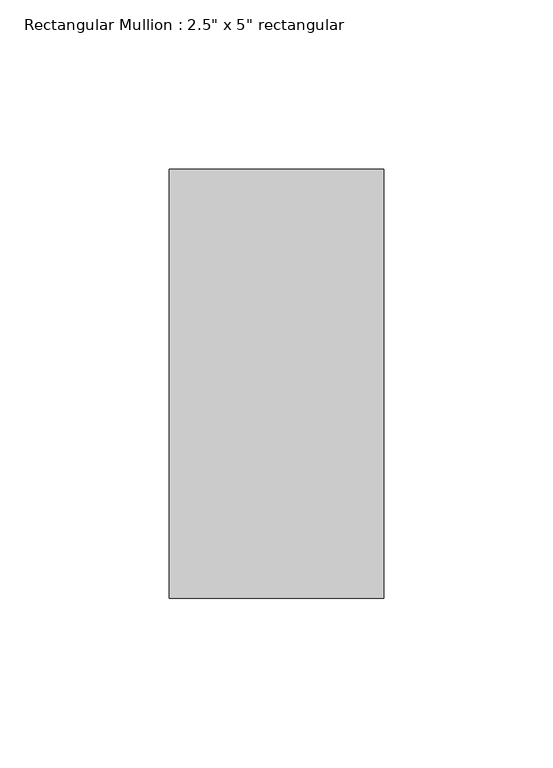
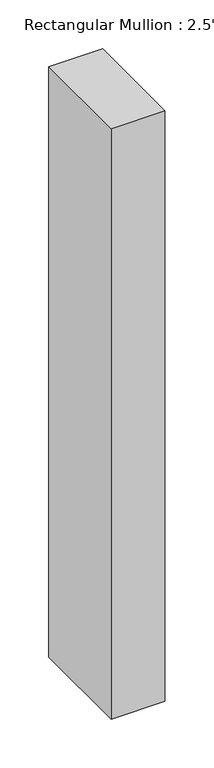
"""IFC4 building model written with IfcOpenShell, lengths in millimetres: member geometry."""

from ifc_helpers import new_model, si_unit, frame, origin, place, context, project, spatial, polyline, outline, extrude, source, transform, mapped, element, save


def member_8ca7f02a(model_context):
    return source(origin(), model_context, "Body", "SweptSolid", [
        extrude(outline(polyline([(31.75, 63.5), (31.75, -63.5), (-31.75, -63.5), (-31.75, 63.5), (31.75, 63.5)])), frame((0.0, 0.0, -736.6), z_axis=(0.0, 0.0, 1.0), x_axis=(1.0, 0.0, 0.0)), (0.0, 0.0, 1.0), 736.6),
    ])


if __name__ == "__main__":
    model = new_model("IFC4")
    model_context = context("Model", 3, world=origin())
    ifc_project = project(units=[si_unit("LENGTHUNIT", "METRE", prefix="MILLI")], contexts=[model_context])
    site = spatial("IfcSite", under=ifc_project)
    building = spatial("IfcBuilding", under=site)
    placement = place(None, origin())
    member_shape = member_8ca7f02a(model_context)
    element("IfcMember", 1, ObjectType="Rectangular Mullion : 2.5\" x 5\" rectangular", at=placement, inside=building, context=model_context, shape_type="MappedRepresentation", body=[
        mapped(member_shape, transform((0.0, 0.0, 0.0), x_axis=(1.0, 0.0, 0.0), y_axis=(0.0, 1.0, 0.0), z_axis=(0.0, 0.0, 1.0))),
    ])
    save(model, "model.ifc")

# Revit data of these elements
# Type "Rectangular Mullion : 2.5\" x 5\" rectangular"
#   built-in parameter 1007304 = 0.416667 (stored number, unit not read)
#   built-in parameter 1007301 = 0.104167 (stored number, unit not read)
#   built-in parameter 1007300 = 0.104167 (stored number, unit not read)
# Element 1 (IfcMember, "Rectangular Mullion : 2.5\" x 5\" rectangular")
#   Materials on its faces: "Aluminum"
# Materials
#   "Aluminum": class "Metal", colour RGB 247 247 247, transparency 0, Description = "Aluminum 6061", Cost = 0
